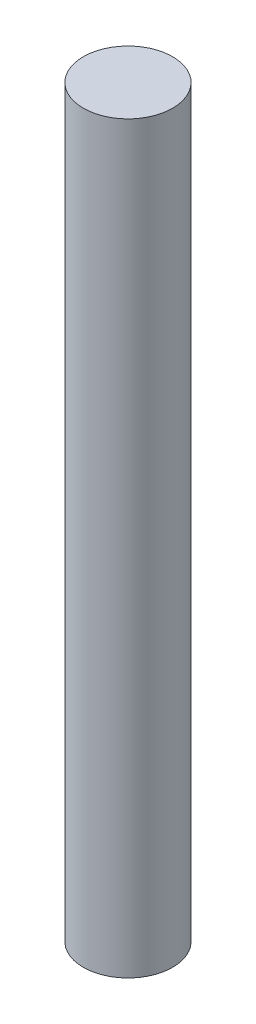
SolidWorks part; units mm, degrees
material "Plain Carbon Steel"
ref_plane "Front Plane" through (0, 0, 0) normal (0, 0, 1) x (1, 0, 0)
ref_plane "Top Plane" through (0, 0, 0) normal (0, 1, 0) x (1, 0, 0)
ref_plane "Right Plane" through (0, 0, 0) normal (1, 0, 0) x (0, 0, -1)
sketch "Shaft Profile Ø24" plane through (0, 0, 0) normal (0, 1, 0) x (1, 0, 0)
  circle A0 centre (0, 0) radius 12
  dimension "D1" = 24
extrude "Shaft Ø24 x 200" add sketch "Shaft Profile Ø24" along normal blind 200
